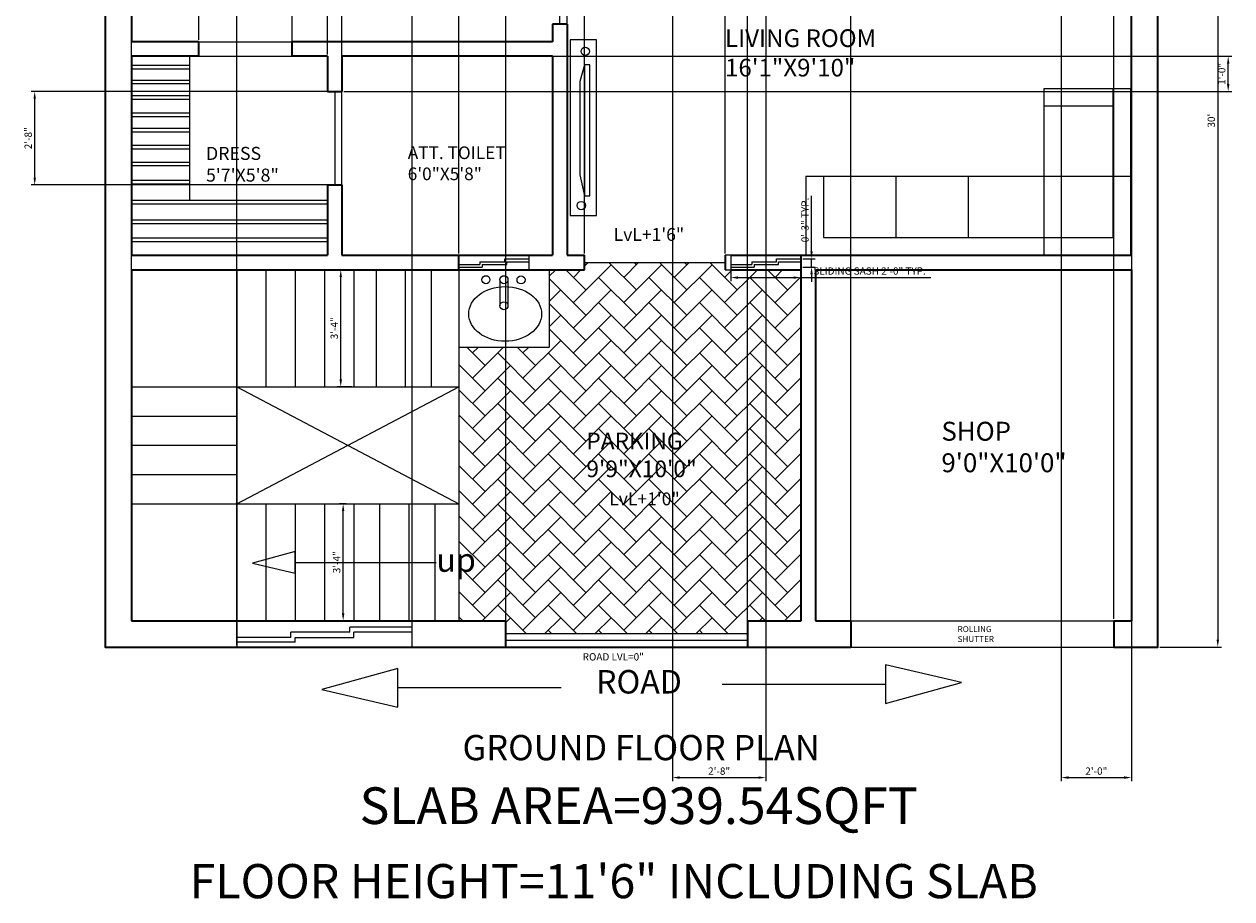
# Model space of a CAD drawing. Units: inches. Extents: x 364 to 777, y 253 to 730.
# Tile 1 of 2: x 364 to 777, y 253 to 552. Entities that reach past the tile are written whole.
import ezdxf

# ---------------------------------------------------------------- set-up
doc = ezdxf.new("R2010")
doc.units = ezdxf.units.IN
for name, color, linetype, lineweight in [('A-ANNO-DIMS', 2, 'Continuous', 18), ('A-ANNO-SYMB', 8, 'Continuous', 18), ('A-ANNO-TEXT', 7, 'Continuous', 25), ('A-AREA-IDEN', 7, 'Continuous', 25), ('A-DOOR', 4, 'Continuous', 18), ('A-EQPM', 8, 'Continuous', 18), ('A-FLOR-CASE', 8, 'Continuous', 18), ('A-FLOR-FIXT', 8, 'Continuous', 18), ('A-FLOR-PATT', 252, 'Continuous', 9), ('A-FLOR-STRS', 7, 'Continuous', 18), ('A-FURN', 8, 'Continuous', 18), ('A-GLAZ', 5, 'Continuous', 18), ('A-WALL', 7, 'Continuous', 35)]:
    doc.layers.add(name, color=color, linetype=linetype, lineweight=lineweight)
doc.styles.get("Standard").update_dxf_attribs({"font": 'arial.ttf'})
doc.dimstyles.new('ISO-25', dxfattribs={"dimtxt": 2.5, "dimasz": 2.5, "dimexe": 1.25, "dimexo": 0.625, "dimtad": 1, "dimdec": 0, "dimlunit": 3, "dimtxsty": 'Standard', "dimcen": 2.5, "dimadec": 0, "dimazin": 0, "dimtfac": 1, "dimtdec": 0, "dimtmove": 0, "dimatfit": 3, "dimfxl": 1, "dimarcsym": 0})

# ---------------------------------------------------------------- blocks, each defined once
blk = doc.blocks.new('*D1')
at = {"layer": 'A-ANNO-DIMS', "color": 0, "lineweight": -2, "transparency": 16777216}
for p, q in [((752.34, 699.12), (773.4, 699.12)), ((772.15, 696.62), (772.15, 341.62)), ((752.34, 339.12), (773.4, 339.12))]:
    blk.add_line(p, q, dxfattribs=at)
at = {"layer": 'A-ANNO-DIMS', "color": 0, "transparency": 16777216}
for points in [[(771.73, 696.62), (772.57, 696.62), (772.15, 699.12)], [(771.73, 341.62), (772.57, 341.62), (772.15, 339.12)]]:
    blk.add_solid(points, dxfattribs=at)
at = {"layer": 'Defpoints', "color": 0, "transparency": 16777216}
for p in [(751.71, 699.12), (751.71, 339.12), (772.15, 339.12)]:
    blk.add_point(p, dxfattribs=at)
at = {"layer": 'A-ANNO-DIMS', "color": 0, "transparency": 16777216, "insert": (770.25, 519.12), "char_height": 2.5, "attachment_point": 5, "rotation": 90}
blk.add_mtext("30'", dxfattribs=at)
blk = doc.blocks.new('*D3')
at = {"layer": 'A-ANNO-DIMS', "color": 0, "lineweight": -2, "transparency": 16777216}
for p, q in [((473.99, 388.12), (471.76, 388.12)), ((473.01, 350.62), (473.01, 385.62)), ((475.99, 348.12), (471.76, 348.12))]:
    blk.add_line(p, q, dxfattribs=at)
at = {"layer": 'A-ANNO-DIMS', "color": 0, "transparency": 16777216}
for points in [[(472.59, 385.62), (473.42, 385.62), (473.01, 388.12)], [(472.59, 350.62), (473.42, 350.62), (473.01, 348.12)]]:
    blk.add_solid(points, dxfattribs=at)
at = {"layer": 'Defpoints', "color": 0, "transparency": 16777216}
for p in [(473.01, 388.12), (474.61, 388.12), (476.61, 348.12)]:
    blk.add_point(p, dxfattribs=at)
at = {"layer": 'A-ANNO-DIMS', "color": 0, "transparency": 16777216, "insert": (471.11, 368.12), "char_height": 2.5, "attachment_point": 5, "rotation": 90}
blk.add_mtext('3\'-4"', dxfattribs=at)
blk = doc.blocks.new('*D4')
at = {"layer": 'A-ANNO-DIMS', "color": 0, "lineweight": -2, "transparency": 16777216}
for p, q in [((475.99, 468.12), (470.94, 468.12)), ((472.19, 430.62), (472.19, 465.62)), ((475.99, 428.12), (470.94, 428.12))]:
    blk.add_line(p, q, dxfattribs=at)
at = {"layer": 'A-ANNO-DIMS', "color": 0, "transparency": 16777216}
for points in [[(471.77, 465.62), (472.6, 465.62), (472.19, 468.12)], [(471.77, 430.62), (472.6, 430.62), (472.19, 428.12)]]:
    blk.add_solid(points, dxfattribs=at)
at = {"layer": 'Defpoints', "color": 0, "transparency": 16777216}
for p in [(472.19, 468.12), (476.61, 468.12), (476.61, 428.12)]:
    blk.add_point(p, dxfattribs=at)
at = {"layer": 'A-ANNO-DIMS', "color": 0, "transparency": 16777216, "insert": (470.28, 448.12), "char_height": 2.5, "attachment_point": 5, "rotation": 90}
blk.add_mtext('3\'-4"', dxfattribs=at)
blk = doc.blocks.new('TV-CONSOLE-60')
for p, q in [((4.94, 51.53), (3.29, 45.83)), ((3.29, 45.83), (3.29, 13.89)), ((3.29, 13.89), (4.94, 6.65))]:
    blk.add_line(p, q)
for points in [[(9, 0), (9, 60), (0, 60), (0, 0)], [(4.94, 6.65), (6.81, 6.65), (6.81, 51.53), (4.94, 51.53)]]:
    blk.add_lwpolyline(points, close=True)
for centre in [(5.17, 56.08), (3.81, 3.36)]:
    blk.add_circle(centre, 1.42)
blk = doc.blocks.new('WIN-SLIDING-SASH-24')
for p, q in [((0, 0.92), (7.14, 0.92)), ((7.14, 1.82), (15.67, 1.82)), ((7.14, 1.82), (7.14, 0.92)), ((7.94, 0.92), (7.94, 0)), ((7.94, 0.92), (16.34, 0.92)), ((15.67, 1.82), (15.67, 2.86)), ((15.67, 2.86), (24, 2.86)), ((16.34, 0.92), (16.34, 1.82)), ((16.34, 1.82), (24, 1.82)), ((0, 0), (7.94, 0))]:
    blk.add_line(p, q)
blk = doc.blocks.new('ARROW-ROAD')
for p, q in [((81.86, 7.15), (55.87, 13.22)), ((55.87, 13.22), (55.87, 0)), ((0, 6.61), (55.87, 6.61)), ((55.87, 0), (81.86, 7.15))]:
    blk.add_line(p, q)
blk = doc.blocks.new('*D16')
at = {"layer": 'A-ANNO-DIMS', "color": 0, "lineweight": -2, "transparency": 16777216}
for p, q in [((605.61, 468.43), (605.61, 464.2)), ((629.61, 468.43), (629.61, 464.2)), ((608.11, 465.45), (627.11, 465.45)), ((629.61, 465.45), (674.01, 465.45))]:
    blk.add_line(p, q, dxfattribs=at)
at = {"layer": 'A-ANNO-DIMS', "color": 0, "transparency": 16777216}
for points in [[(608.11, 465.87), (608.11, 465.03), (605.61, 465.45)], [(627.11, 465.87), (627.11, 465.03), (629.61, 465.45)]]:
    blk.add_solid(points, dxfattribs=at)
at = {"layer": 'Defpoints', "color": 0, "transparency": 16777216}
for p in [(605.61, 469.05), (629.61, 469.05), (629.61, 465.45)]:
    blk.add_point(p, dxfattribs=at)
at = {"layer": 'A-ANNO-DIMS', "color": 0, "transparency": 16777216, "insert": (653.06, 467.37), "char_height": 2.5, "attachment_point": 5}
blk.add_mtext('SLIDING SASH 2\'-0" TYP.', dxfattribs=at)
blk = doc.blocks.new('*D17')
at = {"layer": 'A-ANNO-DIMS', "color": 0, "lineweight": -2, "transparency": 16777216}
for p, q in [((633.21, 474.41), (633.21, 493.4)), ((630.24, 471.91), (634.46, 471.91)), ((633.21, 469.05), (633.21, 471.91)), ((630.24, 469.05), (634.46, 469.05)), ((633.21, 466.55), (633.21, 464.05))]:
    blk.add_line(p, q, dxfattribs=at)
at = {"layer": 'A-ANNO-DIMS', "color": 0, "transparency": 16777216}
for points in [[(632.8, 474.41), (633.63, 474.41), (633.21, 471.91)], [(632.8, 466.55), (633.63, 466.55), (633.21, 469.05)]]:
    blk.add_solid(points, dxfattribs=at)
at = {"layer": 'Defpoints', "color": 0, "transparency": 16777216}
for p in [(629.61, 471.91), (633.21, 471.91), (629.61, 469.05)]:
    blk.add_point(p, dxfattribs=at)
at = {"layer": 'A-ANNO-DIMS', "color": 0, "transparency": 16777216, "insert": (631.31, 485.15), "char_height": 2.5, "attachment_point": 5, "rotation": 90}
blk.add_mtext('0\'-3" TYP.', dxfattribs=at)
blk = doc.blocks.new('*D19')
at = {"layer": 'A-ANNO-DIMS', "color": 0, "lineweight": -2, "transparency": 16777216}
for p, q in [((471.99, 529.1), (366.26, 529.1)), ((367.51, 499.62), (367.51, 526.6)), ((471.99, 497.12), (366.26, 497.12))]:
    blk.add_line(p, q, dxfattribs=at)
at = {"layer": 'A-ANNO-DIMS', "color": 0, "transparency": 16777216}
for points in [[(367.1, 526.6), (367.93, 526.6), (367.51, 529.1)], [(367.1, 499.62), (367.93, 499.62), (367.51, 497.12)]]:
    blk.add_solid(points, dxfattribs=at)
at = {"layer": 'Defpoints', "color": 0, "transparency": 16777216}
for p in [(367.51, 529.1), (472.61, 529.1), (472.61, 497.12)]:
    blk.add_point(p, dxfattribs=at)
at = {"layer": 'A-ANNO-DIMS', "color": 0, "transparency": 16777216, "insert": (365.61, 513.11), "char_height": 2.5, "attachment_point": 5, "rotation": 90}
blk.add_mtext('2\'-8"', dxfattribs=at)
blk = doc.blocks.new('*D21')
at = {"layer": 'A-ANNO-DIMS', "color": 0, "lineweight": -2, "transparency": 16777216}
for p, q in [((391.61, 339.74), (391.61, 724.47)), ((394.11, 723.22), (434.11, 723.22)), ((436.61, 339.74), (436.61, 724.47))]:
    blk.add_line(p, q, dxfattribs=at)
at = {"layer": 'A-ANNO-DIMS', "color": 0, "transparency": 16777216}
for points in [[(394.11, 723.64), (394.11, 722.8), (391.61, 723.22)], [(434.11, 723.64), (434.11, 722.8), (436.61, 723.22)]]:
    blk.add_solid(points, dxfattribs=at)
at = {"layer": 'Defpoints', "color": 0, "transparency": 16777216}
for p in [(436.61, 723.22), (391.61, 339.12), (436.61, 339.12)]:
    blk.add_point(p, dxfattribs=at)
at = {"layer": 'A-ANNO-DIMS', "color": 0, "transparency": 16777216, "insert": (414.11, 725.12), "char_height": 2.5, "attachment_point": 5}
blk.add_mtext('3\'-9"', dxfattribs=at)
blk = doc.blocks.new('*D22')
at = {"layer": 'A-ANNO-DIMS', "color": 0, "lineweight": -2, "transparency": 16777216}
for p, q in [((436.61, 348.74), (436.61, 724.47)), ((439.11, 723.22), (494.11, 723.22)), ((496.61, 348.74), (496.61, 724.47))]:
    blk.add_line(p, q, dxfattribs=at)
at = {"layer": 'A-ANNO-DIMS', "color": 0, "transparency": 16777216}
for points in [[(439.11, 723.64), (439.11, 722.8), (436.61, 723.22)], [(494.11, 723.64), (494.11, 722.8), (496.61, 723.22)]]:
    blk.add_solid(points, dxfattribs=at)
at = {"layer": 'Defpoints', "color": 0, "transparency": 16777216}
for p in [(496.61, 723.22), (436.61, 348.12), (496.61, 348.12)]:
    blk.add_point(p, dxfattribs=at)
at = {"layer": 'A-ANNO-DIMS', "color": 0, "transparency": 16777216, "insert": (466.61, 725.12), "char_height": 2.5, "attachment_point": 5}
blk.add_mtext('5\'-0"', dxfattribs=at)
blk = doc.blocks.new('*D23')
at = {"layer": 'A-ANNO-DIMS', "color": 0, "lineweight": -2, "transparency": 16777216}
for p, q in [((496.61, 339.74), (496.61, 724.47)), ((499.11, 723.22), (526.11, 723.22)), ((528.61, 339.74), (528.61, 724.47))]:
    blk.add_line(p, q, dxfattribs=at)
at = {"layer": 'A-ANNO-DIMS', "color": 0, "transparency": 16777216}
for points in [[(499.11, 723.64), (499.11, 722.8), (496.61, 723.22)], [(526.11, 723.64), (526.11, 722.8), (528.61, 723.22)]]:
    blk.add_solid(points, dxfattribs=at)
at = {"layer": 'Defpoints', "color": 0, "transparency": 16777216}
for p in [(528.61, 723.22), (496.61, 339.12), (528.61, 339.12)]:
    blk.add_point(p, dxfattribs=at)
at = {"layer": 'A-ANNO-DIMS', "color": 0, "transparency": 16777216, "insert": (512.61, 725.12), "char_height": 2.5, "attachment_point": 5}
blk.add_mtext('2\'-8"', dxfattribs=at)
blk = doc.blocks.new('*D24')
at = {"layer": 'A-ANNO-DIMS', "color": 0, "lineweight": -2, "transparency": 16777216}
for p, q in [((528.61, 348.74), (528.61, 724.47)), ((531.11, 723.22), (608.76, 723.22)), ((611.26, 348.74), (611.26, 724.47))]:
    blk.add_line(p, q, dxfattribs=at)
at = {"layer": 'A-ANNO-DIMS', "color": 0, "transparency": 16777216}
for points in [[(531.11, 723.64), (531.11, 722.8), (528.61, 723.22)], [(608.76, 723.64), (608.76, 722.8), (611.26, 723.22)]]:
    blk.add_solid(points, dxfattribs=at)
at = {"layer": 'Defpoints', "color": 0, "transparency": 16777216}
for p in [(611.26, 723.22), (528.61, 348.12), (611.26, 348.12)]:
    blk.add_point(p, dxfattribs=at)
at = {"layer": 'A-ANNO-DIMS', "color": 0, "transparency": 16777216, "insert": (569.94, 725.14), "char_height": 2.5, "attachment_point": 5}
blk.add_mtext('6\'-10 1/2"', dxfattribs=at)
blk = doc.blocks.new('*D25')
at = {"layer": 'A-ANNO-DIMS', "color": 0, "lineweight": -2, "transparency": 16777216}
for p, q in [((611.26, 339.74), (611.26, 724.47)), ((613.76, 723.22), (644.11, 723.22)), ((646.61, 339.74), (646.61, 724.47))]:
    blk.add_line(p, q, dxfattribs=at)
at = {"layer": 'A-ANNO-DIMS', "color": 0, "transparency": 16777216}
for points in [[(613.76, 723.64), (613.76, 722.8), (611.26, 723.22)], [(644.11, 723.64), (644.11, 722.8), (646.61, 723.22)]]:
    blk.add_solid(points, dxfattribs=at)
at = {"layer": 'Defpoints', "color": 0, "transparency": 16777216}
for p in [(646.61, 723.22), (611.26, 339.12), (646.61, 339.12)]:
    blk.add_point(p, dxfattribs=at)
at = {"layer": 'A-ANNO-DIMS', "color": 0, "transparency": 16777216, "insert": (628.94, 725.14), "char_height": 2.5, "attachment_point": 5}
blk.add_mtext('2\'-11 1/2"', dxfattribs=at)
blk = doc.blocks.new('*D26')
at = {"layer": 'A-ANNO-DIMS', "color": 0, "lineweight": -2, "transparency": 16777216}
for p, q in [((646.61, 348.74), (646.61, 724.47)), ((649.11, 723.22), (734.11, 723.22)), ((736.61, 348.74), (736.61, 724.47))]:
    blk.add_line(p, q, dxfattribs=at)
at = {"layer": 'A-ANNO-DIMS', "color": 0, "transparency": 16777216}
for points in [[(649.11, 723.64), (649.11, 722.8), (646.61, 723.22)], [(734.11, 723.64), (734.11, 722.8), (736.61, 723.22)]]:
    blk.add_solid(points, dxfattribs=at)
at = {"layer": 'Defpoints', "color": 0, "transparency": 16777216}
for p in [(736.61, 723.22), (646.61, 348.12), (736.61, 348.12)]:
    blk.add_point(p, dxfattribs=at)
at = {"layer": 'A-ANNO-DIMS', "color": 0, "transparency": 16777216, "insert": (691.61, 725.12), "char_height": 2.5, "attachment_point": 5}
blk.add_mtext('7\'-6"', dxfattribs=at)
blk = doc.blocks.new('*D29')
at = {"layer": 'A-ANNO-DIMS', "color": 0, "lineweight": -2, "transparency": 16777216}
for p, q in [((455.62, 541.74), (455.62, 724.47)), ((458.12, 723.22), (465.11, 723.22)), ((467.61, 541.74), (467.61, 724.47))]:
    blk.add_line(p, q, dxfattribs=at)
at = {"layer": 'A-ANNO-DIMS', "color": 0, "transparency": 16777216}
for points in [[(458.12, 723.64), (458.12, 722.8), (455.62, 723.22)], [(465.11, 723.64), (465.11, 722.8), (467.61, 723.22)]]:
    blk.add_solid(points, dxfattribs=at)
at = {"layer": 'Defpoints', "color": 0, "transparency": 16777216}
for p in [(467.61, 723.22), (455.62, 541.12), (467.61, 541.12)]:
    blk.add_point(p, dxfattribs=at)
at = {"layer": 'A-ANNO-DIMS', "color": 0, "transparency": 16777216, "insert": (461.62, 725.12), "char_height": 2.5, "attachment_point": 5}
blk.add_mtext('1\'-0"', dxfattribs=at)
blk = doc.blocks.new('*D30')
at = {"layer": 'A-ANNO-DIMS', "color": 0, "lineweight": -2, "transparency": 16777216}
for p, q in [((423.62, 546.74), (423.62, 724.47)), ((426.12, 723.22), (453.12, 723.22)), ((455.62, 546.74), (455.62, 724.47))]:
    blk.add_line(p, q, dxfattribs=at)
at = {"layer": 'A-ANNO-DIMS', "color": 0, "transparency": 16777216}
for points in [[(426.12, 723.64), (426.12, 722.8), (423.62, 723.22)], [(453.12, 723.64), (453.12, 722.8), (455.62, 723.22)]]:
    blk.add_solid(points, dxfattribs=at)
at = {"layer": 'Defpoints', "color": 0, "transparency": 16777216}
for p in [(455.62, 723.22), (423.62, 546.12), (455.62, 546.12)]:
    blk.add_point(p, dxfattribs=at)
at = {"layer": 'A-ANNO-DIMS', "color": 0, "transparency": 16777216, "insert": (439.62, 725.12), "char_height": 2.5, "attachment_point": 5}
blk.add_mtext('2\'-8"', dxfattribs=at)
blk = doc.blocks.new('*D31')
at = {"layer": 'A-ANNO-DIMS', "color": 0, "lineweight": -2, "transparency": 16777216}
for p, q in [((585.61, 590.49), (585.61, 293.23)), ((617.61, 590.49), (617.61, 293.23)), ((588.11, 294.48), (615.11, 294.48))]:
    blk.add_line(p, q, dxfattribs=at)
at = {"layer": 'A-ANNO-DIMS', "color": 0, "transparency": 16777216}
for points in [[(588.11, 294.9), (588.11, 294.06), (585.61, 294.48)], [(615.11, 294.9), (615.11, 294.06), (617.61, 294.48)]]:
    blk.add_solid(points, dxfattribs=at)
at = {"layer": 'Defpoints', "color": 0, "transparency": 16777216}
for p in [(585.61, 591.12), (617.61, 591.12), (617.61, 294.48)]:
    blk.add_point(p, dxfattribs=at)
at = {"layer": 'A-ANNO-DIMS', "color": 0, "transparency": 16777216, "insert": (601.61, 296.38), "char_height": 2.5, "attachment_point": 5}
blk.add_mtext('2\'-8"', dxfattribs=at)
blk = doc.blocks.new('*D32')
at = {"layer": 'A-ANNO-DIMS', "color": 0, "lineweight": -2, "transparency": 16777216}
for p, q in [((555.61, 473.74), (555.61, 724.47)), ((558.11, 723.22), (601.21, 723.22)), ((603.71, 473.74), (603.71, 724.47))]:
    blk.add_line(p, q, dxfattribs=at)
at = {"layer": 'A-ANNO-DIMS', "color": 0, "transparency": 16777216}
for points in [[(558.11, 723.64), (558.11, 722.8), (555.61, 723.22)], [(601.21, 723.64), (601.21, 722.8), (603.71, 723.22)]]:
    blk.add_solid(points, dxfattribs=at)
at = {"layer": 'Defpoints', "color": 0, "transparency": 16777216}
for p in [(603.71, 723.22), (555.61, 473.12), (603.71, 473.12)]:
    blk.add_point(p, dxfattribs=at)
at = {"layer": 'A-ANNO-DIMS', "color": 0, "transparency": 16777216, "insert": (579.66, 725.12), "char_height": 2.5, "attachment_point": 5}
blk.add_mtext('4\'-0"', dxfattribs=at)
blk = doc.blocks.new('*D33')
at = {"layer": 'A-ANNO-DIMS', "color": 0, "lineweight": -2, "transparency": 16777216}
for p, q in [((473.24, 541.12), (776.96, 541.12)), ((775.71, 531.6), (775.71, 538.62)), ((473.24, 529.1), (776.96, 529.1))]:
    blk.add_line(p, q, dxfattribs=at)
at = {"layer": 'A-ANNO-DIMS', "color": 0, "transparency": 16777216}
for points in [[(775.3, 538.62), (776.13, 538.62), (775.71, 541.12)], [(775.3, 531.6), (776.13, 531.6), (775.71, 529.1)]]:
    blk.add_solid(points, dxfattribs=at)
at = {"layer": 'Defpoints', "color": 0, "transparency": 16777216}
for p in [(472.61, 541.12), (775.71, 541.12), (472.61, 529.1)]:
    blk.add_point(p, dxfattribs=at)
at = {"layer": 'A-ANNO-DIMS', "color": 0, "transparency": 16777216, "insert": (773.81, 535.11), "char_height": 2.5, "attachment_point": 5, "rotation": 90}
blk.add_mtext('1\'-0"', dxfattribs=at)
blk = doc.blocks.new('*D34')
at = {"layer": 'A-ANNO-DIMS', "color": 0, "lineweight": -2, "transparency": 16777216}
for p, q in [((718.61, 590.49), (718.61, 293.23)), ((742.61, 590.49), (742.61, 293.23)), ((721.11, 294.48), (740.11, 294.48))]:
    blk.add_line(p, q, dxfattribs=at)
at = {"layer": 'A-ANNO-DIMS', "color": 0, "transparency": 16777216}
for points in [[(721.11, 294.9), (721.11, 294.06), (718.61, 294.48)], [(740.11, 294.9), (740.11, 294.06), (742.61, 294.48)]]:
    blk.add_solid(points, dxfattribs=at)
at = {"layer": 'Defpoints', "color": 0, "transparency": 16777216}
for p in [(718.61, 591.12), (742.61, 591.12), (742.61, 294.48)]:
    blk.add_point(p, dxfattribs=at)
at = {"layer": 'A-ANNO-DIMS', "color": 0, "transparency": 16777216, "insert": (730.61, 296.38), "char_height": 2.5, "attachment_point": 5}
blk.add_mtext('2\'-0"', dxfattribs=at)
blk = doc.blocks.new('*D35')
at = {"layer": 'A-ANNO-DIMS', "color": 0, "lineweight": -2, "transparency": 16777216}
for p, q in [((400.61, 428.74), (400.61, 724.47)), ((403.11, 723.22), (434.11, 723.22)), ((436.61, 428.74), (436.61, 724.47))]:
    blk.add_line(p, q, dxfattribs=at)
at = {"layer": 'A-ANNO-DIMS', "color": 0, "transparency": 16777216}
for points in [[(403.11, 723.64), (403.11, 722.8), (400.61, 723.22)], [(434.11, 723.64), (434.11, 722.8), (436.61, 723.22)]]:
    blk.add_solid(points, dxfattribs=at)
at = {"layer": 'Defpoints', "color": 0, "transparency": 16777216}
for p in [(436.61, 723.22), (400.61, 428.12), (436.61, 428.12)]:
    blk.add_point(p, dxfattribs=at)
at = {"layer": 'A-ANNO-DIMS', "color": 0, "transparency": 16777216, "insert": (418.61, 725.12), "char_height": 2.5, "attachment_point": 5}
blk.add_mtext('3\'-0"', dxfattribs=at)
blk = doc.blocks.new('*D36')
at = {"layer": 'A-ANNO-DIMS', "color": 0, "lineweight": -2, "transparency": 16777216}
for p, q in [((472.61, 473.74), (472.61, 724.47)), ((475.11, 723.22), (510.11, 723.22)), ((512.61, 473.74), (512.61, 724.47))]:
    blk.add_line(p, q, dxfattribs=at)
at = {"layer": 'A-ANNO-DIMS', "color": 0, "transparency": 16777216}
for points in [[(475.11, 723.64), (475.11, 722.8), (472.61, 723.22)], [(510.11, 723.64), (510.11, 722.8), (512.61, 723.22)]]:
    blk.add_solid(points, dxfattribs=at)
at = {"layer": 'Defpoints', "color": 0, "transparency": 16777216}
for p in [(512.61, 723.22), (472.61, 473.12), (512.61, 473.12)]:
    blk.add_point(p, dxfattribs=at)
at = {"layer": 'A-ANNO-DIMS', "color": 0, "transparency": 16777216, "insert": (492.61, 725.12), "char_height": 2.5, "attachment_point": 5}
blk.add_mtext('3\'-4"', dxfattribs=at)
blk = doc.blocks.new('*D37')
at = {"layer": 'A-ANNO-DIMS', "color": 0, "lineweight": -2, "transparency": 16777216}
for p, q in [((547.11, 723.22), (544.61, 723.22)), ((549.61, 473.74), (549.61, 724.47)), ((549.61, 723.22), (555.61, 723.22)), ((555.61, 473.74), (555.61, 724.47)), ((558.11, 723.22), (568.51, 723.22))]:
    blk.add_line(p, q, dxfattribs=at)
at = {"layer": 'A-ANNO-DIMS', "color": 0, "transparency": 16777216}
for points in [[(547.11, 723.64), (547.11, 722.8), (549.61, 723.22)], [(558.11, 723.64), (558.11, 722.8), (555.61, 723.22)]]:
    blk.add_solid(points, dxfattribs=at)
at = {"layer": 'Defpoints', "color": 0, "transparency": 16777216}
for p in [(555.61, 723.22), (549.61, 473.12), (555.61, 473.12)]:
    blk.add_point(p, dxfattribs=at)
at = {"layer": 'A-ANNO-DIMS', "color": 0, "transparency": 16777216, "insert": (564.56, 725.12), "char_height": 2.5, "attachment_point": 5}
blk.add_mtext('0\'-6"', dxfattribs=at)

msp = doc.modelspace()

# ---------------------------------------------------------------- hatches: boundary and pattern name
at = {"layer": 'A-FLOR-PATT'}
h = msp.add_hatch(dxfattribs=at)
h.set_pattern_fill('AR-HBONE', color=256, scale=0.06)
h.paths.add_polyline_path([(629.61, 468.12), (603.71, 468.12), (603.71, 470.62), (555.61, 470.62), (555.61, 468.12), (543.49, 468.12), (543.49, 441.69), (512.61, 441.69), (512.61, 348.12), (528.61, 348.12), (528.61, 343.62), (611.26, 343.62), (611.26, 348.12), (629.61, 348.12)])
h.paths.add_polyline_path([(502.1, 360.43), (518.73, 360.43), (518.73, 377.12), (502.1, 377.12)], flags=9)
h.paths.add_polyline_path([(562.85, 386.86), (582.29, 386.86), (582.29, 393.66), (562.85, 393.66)], flags=24)
h.paths.add_polyline_path([(554.15, 393.97), (593.47, 393.97), (593.47, 415.26), (554.15, 415.26)], flags=24)

# ---------------------------------------------------------------- linework, layer by layer
at = {"layer": 'A-ANNO-SYMB'}
for p, q in [((456.6, 371.77), (442.05, 367.77)), ((456.6, 364.37), (456.6, 371.77)), ((442.05, 367.77), (456.6, 364.37)), ((456.6, 368.07), (504.85, 368.07))]:
    msp.add_line(p, q, dxfattribs=at)
at = {"layer": 'A-DOOR'}
for p, q in [((547.11, 552.12), (547.11, 591.12)), ((423.62, 546.12), (455.62, 546.12)), ((423.62, 541.12), (455.62, 541.12)), ((470.11, 529.12), (470.11, 497.12)), ((555.61, 470.62), (603.71, 470.62)), ((646.61, 348.12), (736.61, 348.12)), ((611.26, 343.62), (528.61, 343.62)), ((611.26, 341.39), (528.61, 341.39)), ((646.61, 339.12), (736.61, 339.12))]:
    msp.add_line(p, q, dxfattribs=at)
at = {"layer": 'A-FLOR-CASE'}
for p, q in [((420.42, 541.12), (420.42, 491.94)), ((400.61, 538.13), (420.42, 538.13)), ((400.61, 536.89), (420.42, 536.89)), ((400.61, 533.01), (420.42, 533.01)), ((400.61, 531.77), (420.42, 531.77)), ((400.61, 527.72), (420.42, 527.72)), ((400.61, 526.48), (420.42, 526.48)), ((400.61, 521.82), (420.42, 521.82)), ((400.61, 520.57), (420.42, 520.57)), ((400.61, 516.53), (420.42, 516.53)), ((400.61, 515.29), (420.42, 515.29)), ((400.61, 510.71), (420.42, 510.71)), ((400.61, 509.47), (420.42, 509.47)), ((400.61, 504.98), (420.42, 504.98)), ((400.61, 503.74), (420.42, 503.74)), ((400.61, 498.81), (420.42, 498.81)), ((400.61, 497.56), (420.42, 497.56)), ((400.61, 491.94), (420.42, 491.94)), ((420.42, 491.94), (467.61, 491.94)), ((400.61, 490.7), (467.61, 490.7)), ((400.61, 485.21), (467.61, 485.21)), ((400.61, 483.97), (467.61, 483.97)), ((400.61, 479.03), (467.61, 479.03)), ((400.61, 477.79), (467.61, 477.79))]:
    msp.add_line(p, q, dxfattribs=at)
at = {"layer": 'A-FLOR-FIXT'}
for p, q in [((543.49, 468.12), (543.49, 441.69)), ((526.65, 464.74), (526.65, 455.83)), ((529.39, 464.74), (529.39, 455.83)), ((512.61, 441.69), (543.49, 441.69))]:
    msp.add_line(p, q, dxfattribs=at)
for centre in [(521.85, 464.74), (528.02, 464.74), (533.84, 464.67), (528.02, 455.84)]:
    msp.add_circle(centre, 1.37, dxfattribs=at)
msp.add_ellipse((528.41, 453.03), major_axis=(12.45, 0), ratio=0.751725, dxfattribs=at)
at = {"layer": 'A-FLOR-STRS'}
for p, q in [((436.61, 468.12), (436.61, 388.12)), ((446.61, 468.12), (446.61, 428.12)), ((456.61, 468.12), (456.61, 428.12)), ((466.61, 468.12), (466.61, 428.12)), ((476.61, 468.12), (476.61, 428.12)), ((484.26, 468.12), (484.26, 428.12)), ((494.26, 468.12), (494.26, 428.12)), ((503.15, 468.12), (503.15, 428.12)), ((512.61, 468.12), (512.61, 348.12)), ((400.61, 428.12), (512.61, 428.12)), ((436.61, 388.12), (512.61, 428.12)), ((436.61, 428.12), (512.61, 388.12)), ((400.61, 418.12), (436.61, 418.12)), ((400.61, 408.12), (436.61, 408.12)), ((400.61, 398.12), (436.61, 398.12)), ((400.61, 388.12), (436.61, 388.12)), ((436.61, 388.12), (436.61, 348.12)), ((436.61, 388.12), (512.61, 388.12)), ((446.61, 388.12), (446.61, 348.12)), ((456.61, 388.12), (456.61, 348.12)), ((466.61, 388.12), (466.61, 348.12)), ((476.61, 388.12), (476.61, 348.12)), ((485.43, 388.12), (485.43, 348.12)), ((495.43, 388.12), (495.43, 348.12)), ((504.34, 388.12), (504.34, 348.12))]:
    msp.add_line(p, q, dxfattribs=at)
at = {"layer": 'A-FURN'}
for p, q in [((712.78, 473.12), (712.78, 530.16)), ((712.78, 530.16), (742.36, 530.16)), ((736.36, 479.12), (736.36, 530.16)), ((742.36, 473.12), (742.36, 530.16)), ((712.78, 524.16), (736.36, 524.16)), ((631.25, 500.13), (631.25, 473.12)), ((631.25, 500.13), (742.36, 500.13)), ((637.25, 500.13), (637.25, 479.12)), ((662.08, 500.13), (662.08, 479.12)), ((686.8, 500.13), (686.8, 479.12)), ((637.25, 479.12), (736.36, 479.12)), ((631.25, 473.12), (742.36, 473.12))]:
    msp.add_line(p, q, dxfattribs=at)
at = {"layer": 'A-GLAZ'}
for p, q in [((629.61, 473.12), (603.71, 473.12)), ((605.61, 473.12), (605.61, 468.12)), ((629.61, 468.12), (629.61, 473.12)), ((603.71, 468.12), (629.61, 468.12)), ((436.61, 348.12), (436.61, 339.12)), ((496.61, 348.12), (436.61, 348.12)), ((496.61, 339.12), (496.61, 348.12)), ((455.17, 342.37), (455.17, 344.21)), ((475.34, 344.18), (455.17, 344.18)), ((496.61, 345.9), (475.34, 345.9)), ((475.34, 344.18), (475.34, 345.9)), ((496.61, 344.18), (476.68, 344.18)), ((476.68, 342.41), (476.68, 344.18)), ((455.17, 342.37), (436.61, 342.37)), ((456.63, 340.79), (436.61, 340.79)), ((436.61, 339.12), (496.61, 339.12)), ((456.63, 342.37), (476.68, 342.41)), ((456.63, 340.79), (456.63, 342.37))]:
    msp.add_line(p, q, dxfattribs=at)
msp.add_lwpolyline([(512.61, 468.12), (536.61, 468.12), (536.61, 473.12), (512.61, 473.12)], close=True, dxfattribs=at)
at = {"layer": 'A-WALL'}
for p, q in [((400.61, 690.12), (400.61, 546.12)), ((742.61, 473.12), (742.61, 690.12)), ((549.61, 552.12), (544.61, 552.12)), ((544.61, 552.12), (544.61, 546.12)), ((549.61, 552.12), (549.61, 473.12)), ((423.62, 546.12), (400.61, 546.12)), ((423.62, 541.12), (423.62, 546.12)), ((544.61, 546.12), (455.62, 546.12)), ((455.62, 541.12), (455.62, 546.12)), ((400.61, 541.12), (400.61, 473.12)), ((423.62, 541.12), (400.61, 541.12)), ((467.61, 541.12), (455.62, 541.12)), ((467.61, 541.12), (467.61, 529.14)), ((544.61, 541.12), (472.61, 541.12)), ((472.61, 541.12), (472.61, 529.1)), ((544.61, 541.12), (544.61, 473.12)), ((467.61, 529.14), (472.61, 529.1)), ((467.61, 497.12), (472.61, 497.12)), ((467.61, 497.12), (467.61, 473.12)), ((472.61, 497.12), (472.61, 473.12)), ((400.61, 473.12), (467.61, 473.12)), ((472.61, 473.12), (544.61, 473.12)), ((512.61, 468.12), (512.61, 473.12)), ((549.61, 473.12), (555.61, 473.12)), ((555.61, 468.12), (555.61, 473.12)), ((603.71, 473.12), (603.71, 468.12)), ((605.61, 473.12), (742.61, 473.12)), ((629.61, 468.12), (629.61, 473.12)), ((400.61, 468.12), (512.61, 468.12)), ((400.61, 468.12), (400.61, 348.12)), ((512.61, 468.12), (555.61, 468.12)), ((605.61, 468.12), (629.61, 468.12)), ((629.61, 348.12), (629.61, 468.12)), ((634.61, 468.12), (742.61, 468.12)), ((634.61, 468.12), (634.61, 348.12)), ((742.61, 468.12), (742.61, 348.12)), ((400.61, 348.12), (512.61, 348.12)), ((512.61, 348.12), (528.61, 348.12)), ((528.61, 339.12), (528.61, 348.12)), ((611.26, 348.12), (611.26, 339.12)), ((611.26, 348.12), (629.61, 348.12)), ((634.61, 348.12), (634.61, 348.12)), ((634.61, 348.12), (646.61, 348.12)), ((646.61, 348.12), (646.61, 339.12)), ((736.61, 348.12), (736.61, 339.12)), ((736.61, 348.12), (742.61, 348.12))]:
    msp.add_line(p, q, dxfattribs=at)
msp.add_lwpolyline([(736.61, 339.12), (751.61, 339.12), (751.61, 699.12), (391.61, 699.12), (391.61, 339.12), (646.61, 339.12)], dxfattribs=at)

# ---------------------------------------------------------------- block references
at = {"layer": 'A-ANNO-SYMB', "rotation": 180}
msp.add_blockref('ARROW-ROAD', (547.56, 331.8), dxfattribs=at)
at = {"layer": 'A-ANNO-SYMB'}
msp.add_blockref('ARROW-ROAD', (602.66, 319.8), dxfattribs=at)
at = {"layer": 'A-EQPM'}
msp.add_blockref('TV-CONSOLE-60', (550.62, 486.73), dxfattribs=at)
at = {"layer": 'A-GLAZ'}
for p in [(512.61, 469.05), (605.61, 469.05)]:
    msp.add_blockref('WIN-SLIDING-SASH-24', p, dxfattribs=at)

# ---------------------------------------------------------------- texts
at = {"layer": 'A-ANNO-SYMB', "attachment_point": 1}
for s, width, gutter_width, insert, char_height in [('LvL+1\'6"', 31.1824, 21.96, (565.55, 482.4), 4.392), ('LvL+1\'0"', 47.2522, 16.51, (564.02, 391.98), 4.392), ('up', 75.8211, 40.49, (504.85, 372.95), 8.099), ('ROAD LVL=0"', 26.2269, 12.5, (554.92, 337.02), 2.5)]:
    msp.add_mtext_dynamic_manual_height_columns(s, width=width, gutter_width=gutter_width, heights=[0], dxfattribs=dict(at, insert=insert, char_height=char_height))
at = {"layer": 'A-ANNO-TEXT', "attachment_point": 1}
for s, width, gutter_width, insert, char_height in [('ROLLING SHUTTER', 13.2704, 10.22, (683.16, 346.27), 2.043), ('ROAD', 172.2856, 40.17, (559.55, 331.26), 8.035), ('GROUND FLOOR PLAN', 300.8491, 43.2, (513.83, 309.05), 8.6397), ('SLAB AREA=939.54SQFT', 362.6752, 62.68, (478.63, 291.14), 12.5351), ('FLOOR HEIGHT=11\'6" INCLUDING SLAB', 323.1618, 58.43, (420.47, 264.91), 11.6865)]:
    msp.add_mtext_dynamic_manual_height_columns(s, width=width, gutter_width=gutter_width, heights=[0], dxfattribs=dict(at, insert=insert, char_height=char_height))
at = {"layer": 'A-AREA-IDEN', "attachment_point": 1}
for s, width, gutter_width, insert, char_height in [('LIVING ROOM\\P16\'1"X9\'10"', 154.0611, 30.22, (603.62, 550.35), 6.044), ('DRESS\\P5\'7\'X5\'8"', 54.7356, 22.27, (426.1, 510.15), 4.454), ('ATT. TOILET\\P6\'0"X5\'8"', 54.9173, 21.63, (495.1, 510.31), 4.3268), ('SHOP\\P9\'0"X10\'0"', 125.553, 32.34, (677.63, 416.15), 6.468), ('PARKING\\P9\'9"X10\'0"', 145.2306, 28.53, (556.19, 412.42), 5.705)]:
    msp.add_mtext_dynamic_manual_height_columns(s, width=width, gutter_width=gutter_width, heights=[0], dxfattribs=dict(at, insert=insert, char_height=char_height))

# ---------------------------------------------------------------- dimensions: what is measured, and where the dimension line sits
at = {"layer": 'A-ANNO-DIMS'}
for base, p1, p2, picture, middle in [((611.2615, 723.2187), (528.6114, 348.1187), (611.2615, 348.1187), '*D24', (569.9364, 725.1364)), ((646.6117, 723.2187), (611.2615, 339.1187), (646.6117, 339.1187), '*D25', (628.9366, 725.1364)), ((436.61, 723.22), (391.61, 339.12), (436.61, 339.12), '*D21', (414.11, 725.12)), ((436.61, 723.22), (400.61, 428.12), (436.61, 428.12), '*D35', (418.61, 725.12)), ((455.62, 723.22), (423.62, 546.12), (455.62, 546.12), '*D30', (439.62, 725.12)), ((496.61, 723.22), (436.61, 348.12), (496.61, 348.12), '*D22', (466.61, 725.12)), ((467.61, 723.22), (455.62, 541.12), (467.61, 541.12), '*D29', (461.62, 725.12)), ((512.61, 723.22), (472.61, 473.12), (512.61, 473.12), '*D36', (492.61, 725.12)), ((528.61, 723.22), (496.61, 339.12), (528.61, 339.12), '*D23', (512.61, 725.12)), ((555.61, 723.22), (549.61, 473.12), (555.61, 473.12), '*D37', (564.56, 725.12)), ((603.71, 723.22), (555.61, 473.12), (603.71, 473.12), '*D32', (579.66, 725.12)), ((736.61, 723.22), (646.61, 348.12), (736.61, 348.12), '*D26', (691.61, 725.12)), ((617.61, 294.48), (585.61, 591.12), (617.61, 591.12), '*D31', (601.61, 296.38)), ((742.61, 294.48), (718.61, 591.12), (742.61, 591.12), '*D34', (730.61, 296.38))]:
    dim = msp.add_linear_dim(base=base, p1=p1, p2=p2, dimstyle='ISO-25', override={"dimdec": 1, "dimlfac": 1, "dimrnd": 0, "dimzin": 1, "dimdsep": 46, "dimlunit": 4, "dimfrac": 2}, dxfattribs=at)
    dim.commit()
    dim.dimension.update_dxf_attribs({"geometry": picture, "text_midpoint": middle})
for base, p1, p2, override, picture, middle in [((772.15, 339.12), (751.71, 699.12), (751.71, 339.12), {"dimclrd": 0, "dimclre": 0, "dimclrt": 0}, '*D1', (770.25, 519.12)), ((775.71, 541.12), (472.61, 529.1), (472.61, 541.12), {"dimdec": 1, "dimlfac": 1, "dimrnd": 0, "dimzin": 1, "dimdsep": 46, "dimlunit": 4, "dimfrac": 2}, '*D33', (773.81, 535.11)), ((367.51, 529.1), (472.61, 497.12), (472.61, 529.1), {"dimdec": 1, "dimlfac": 1, "dimrnd": 0, "dimzin": 1, "dimdsep": 46, "dimlunit": 4, "dimfrac": 2}, '*D19', (365.61, 513.11)), ((472.19, 468.12), (476.61, 428.12), (476.61, 468.12), {"dimclrd": 0, "dimclre": 0, "dimclrt": 0}, '*D4', (470.28, 448.12)), ((473.01, 388.12), (476.61, 348.12), (474.61, 388.12), {"dimclrd": 0, "dimclre": 0, "dimclrt": 0}, '*D3', (471.11, 368.12))]:
    dim = msp.add_linear_dim(base=base, p1=p1, p2=p2, angle=90, dimstyle='ISO-25', override=override, dxfattribs=at)
    dim.commit()
    dim.dimension.update_dxf_attribs({"geometry": picture, "text_midpoint": middle})
dim = msp.add_linear_dim(base=(633.21, 471.91), p1=(629.61, 469.05), p2=(629.61, 471.91), angle=90, text='<> TYP.', dimstyle='ISO-25', override={"dimdec": 1, "dimlfac": 1, "dimrnd": 0, "dimzin": 1, "dimdsep": 46, "dimlunit": 4, "dimfrac": 2}, dxfattribs=at)
dim.commit()
dim.dimension.update_dxf_attribs({"geometry": '*D17', "text_midpoint": (631.31, 485.15)})
dim = msp.add_linear_dim(base=(629.61, 465.45), p1=(605.61, 469.05), p2=(629.61, 469.05), text='SLIDING SASH <> TYP.', dimstyle='ISO-25', override={"dimdec": 1, "dimlfac": 1, "dimrnd": 0, "dimzin": 1, "dimdsep": 46, "dimlunit": 4, "dimfrac": 2}, dxfattribs=at)
dim.commit()
dim.dimension.update_dxf_attribs({"geometry": '*D16', "text_midpoint": (653.06, 467.37)})

doc.saveas('drawing.dxf')
